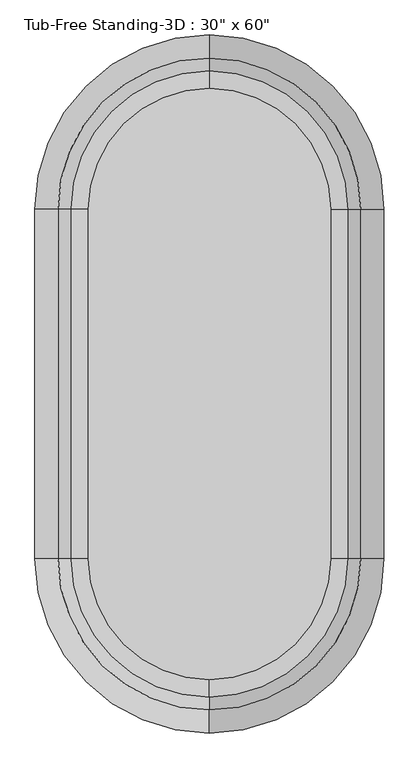
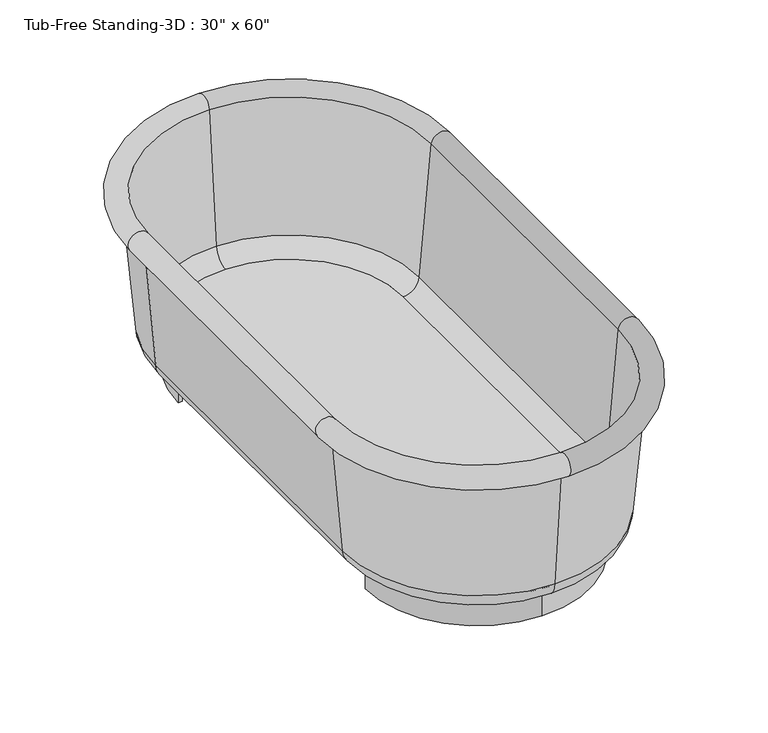
"""IFC4 building model written with IfcOpenShell, lengths in millimetres: flow terminal geometry."""

from ifc_helpers import new_model, si_unit, point, frame, frame_2d, origin, origin_with_axes, place, context, project, spatial, polyline, circle_curve, ellipse_curve, trimmed, segment, composite_curve, outline, extrude, source, transform, mapped, element, save
from ifc_brep_helpers import plane_surface, cylinder_surface, revolved_surface, advanced_brep


def flow_terminal_b374fae2(model_context):
    return source(origin(), model_context, "Body", "SolidModel", [
        extrude(outline(composite_curve([segment(trimmed(circle_curve(frame_2d((0.0, 381.0)), 254.0), [point((0.0, 635.0))], [point((-254.0, 381.0))], True, "CARTESIAN"), True, "CONTINUOUS"), segment(polyline([(-254.0, 381.0), (-264.2824236, 381.0)]), True, "CONTINUOUS"), segment(trimmed(circle_curve(frame_2d((0.0, 381.0)), 264.2824236), [point((-264.2824236, 381.0))], [point((0.0, 645.2824236))], False, "CARTESIAN"), True, "CONTINUOUS"), segment(trimmed(circle_curve(frame_2d((0.0, 381.0)), 264.2824236), [point((0.0, 645.2824236))], [point((264.2824236, 381.0))], False, "CARTESIAN"), True, "CONTINUOUS"), segment(polyline([(264.2824236, 381.0), (254.0, 381.0)]), True, "CONTINUOUS"), segment(trimmed(circle_curve(frame_2d((0.0, 381.0)), 254.0), [point((254.0, 381.0))], [point((0.0, 635.0))], True, "CARTESIAN"), True, "CONTINUOUS")], self_intersect=False)), origin_with_axes(), (0.0, 0.0, 1.0), 63.5),
        extrude(outline(composite_curve([segment(trimmed(circle_curve(frame_2d((0.0, -381.0)), 264.2824236), [point((0.0, -645.2824236))], [point((-264.2824236, -381.0))], False, "CARTESIAN"), True, "CONTINUOUS"), segment(polyline([(-264.2824236, -381.0), (-254.0, -381.0)]), True, "CONTINUOUS"), segment(trimmed(circle_curve(frame_2d((0.0, -381.0)), 254.0), [point((-254.0, -381.0))], [point((0.0, -635.0))], True, "CARTESIAN"), True, "CONTINUOUS"), segment(trimmed(circle_curve(frame_2d((0.0, -381.0)), 254.0), [point((0.0, -635.0))], [point((254.0, -381.0))], True, "CARTESIAN"), True, "CONTINUOUS"), segment(polyline([(254.0, -381.0), (264.2824236, -381.0)]), True, "CONTINUOUS"), segment(trimmed(circle_curve(frame_2d((0.0, -381.0)), 264.2824236), [point((264.2824236, -381.0))], [point((0.0, -645.2824236))], False, "CARTESIAN"), True, "CONTINUOUS")], self_intersect=False)), origin_with_axes(), (0.0, 0.0, 1.0), 63.5),
        extrude(outline(composite_curve([segment(polyline([(-264.2824236, -381.0), (-264.2824236, 381.0)]), True, "CONTINUOUS"), segment(trimmed(circle_curve(frame_2d((0.0, 381.0)), 264.2824236), [point((-264.2824236, 381.0))], [point((0.0, 645.2824236))], False, "CARTESIAN"), True, "CONTINUOUS"), segment(trimmed(circle_curve(frame_2d((0.0, 381.0)), 264.2824236), [point((0.0, 645.2824236))], [point((264.2824236, 381.0))], False, "CARTESIAN"), True, "CONTINUOUS"), segment(polyline([(264.2824236, 381.0), (264.2824236, -381.0)]), True, "CONTINUOUS"), segment(trimmed(circle_curve(frame_2d((0.0, -381.0)), 264.2824236), [point((264.2824236, -381.0))], [point((0.0, -645.2824236))], False, "CARTESIAN"), True, "CONTINUOUS"), segment(trimmed(circle_curve(frame_2d((0.0, -381.0)), 264.2824236), [point((0.0, -645.2824236))], [point((-264.2824236, -381.0))], False, "CARTESIAN"), True, "CONTINUOUS")], self_intersect=False)), frame((0.0, 0.0, 63.5), z_axis=(0.0, 0.0, 1.0), x_axis=(1.0, 0.0, 0.0)), (0.0, 0.0, 1.0), 15.08125),
        advanced_brep(
        [(0.0, -723.9, 406.4), (342.9, -381.0, 406.4), (355.6, -381.0, 406.4), (0.0, -736.6, 406.4), (0.0, -698.1045038, 111.5561295), (317.1045038, -381.0, 111.5561295), (0.0, -645.2824236, 63.1536107), (264.2824236, -381.0, 63.1536107), (0.0, -645.2824236, 78.0774627), (264.2824236, -381.0, 78.0774627), (0.0, -683.2374416, 112.8568289), (302.2374416, -381.0, 112.8568289), (0.0, -711.4561556, 435.3982063), (330.4561556, -381.0, 435.3982063), (-342.9, -381.0, 406.4), (-355.6, -381.0, 406.4), (-317.1045038, -381.0, 111.5561295), (-264.2824236, -381.0, 63.1536107), (-264.2824236, -381.0, 78.0774627), (-302.2374416, -381.0, 112.8568289), (-330.4561556, -381.0, 435.3982063), (-355.6, 381.0, 406.4), (-342.9, 381.0, 406.4), (-317.1045038, 381.0, 111.5561295), (-264.2824236, 381.0, 63.1536107), (-264.2824236, 381.0, 78.0774627), (-302.2374416, 381.0, 112.8568289), (-330.4561556, 381.0, 435.3982063), (0.0, 723.9, 406.4), (0.0, 736.6, 406.4), (0.0, 698.1045038, 111.5561295), (0.0, 645.2824236, 63.1536107), (0.0, 645.2824236, 78.0774627), (0.0, 683.2374416, 112.8568289), (0.0, 711.4561556, 435.3982063), (342.9, 381.0, 406.4), (355.6, 381.0, 406.4), (317.1045038, 381.0, 111.5561295), (264.2824236, 381.0, 63.1536107), (264.2824236, 381.0, 78.0774627), (302.2374416, 381.0, 112.8568289), (330.4561556, 381.0, 435.3982063)],
        [
            (0, 1, circle_curve(frame((0.0, -381.0, 406.4), z_axis=(0.0, 0.0, 1.0), x_axis=(1.0, 0.0, 0.0)), 342.9)),
            (1, 2),
            (2, 3, circle_curve(frame((0.0, -381.0, 406.4), z_axis=(0.0, 0.0, -1.0), x_axis=(1.0, 0.0, 0.0)), 355.6)),
            (3, 0),
            (4, 5, circle_curve(frame((0.0, -381.0, 111.5561295), z_axis=(0.0, 0.0, 1.0), x_axis=(1.0, 0.0, 0.0)), 317.1045038)),
            (5, 1),
            (0, 4),
            (6, 7, circle_curve(frame((0.0, -381.0, 63.1536107), z_axis=(0.0, 0.0, 1.0), x_axis=(1.0, 0.0, 0.0)), 264.2824236)),
            (7, 5, circle_curve(frame((264.2824236, -381.0, 116.1774627), z_axis=(0.0, -1.0, 0.0), x_axis=(1.0, 0.0, 0.0)), 53.023852)),
            (4, 6, circle_curve(frame((0.0, -645.2824236, 116.1774627), z_axis=(1.0, 0.0, 0.0), x_axis=(0.0, -1.0, 0.0)), 53.023852)),
            (8, 9, circle_curve(frame((0.0, -381.0, 78.0774627), z_axis=(0.0, 0.0, 1.0), x_axis=(1.0, 0.0, 0.0)), 264.2824236)),
            (9, 7),
            (6, 8),
            (10, 11, circle_curve(frame((0.0, -381.0, 112.8568289), z_axis=(0.0, 0.0, 1.0), x_axis=(1.0, 0.0, 0.0)), 302.2374416)),
            (11, 9, circle_curve(frame((264.2824236, -381.0, 116.1774627), z_axis=(0.0, 1.0, 0.0), x_axis=(1.0, 0.0, 0.0)), 38.1)),
            (8, 10, circle_curve(frame((0.0, -645.2824236, 116.1774627), z_axis=(-1.0, 0.0, 0.0), x_axis=(0.0, -1.0, 0.0)), 38.1)),
            (12, 13, circle_curve(frame((0.0, -381.0, 435.3982063), z_axis=(0.0, 0.0, 1.0), x_axis=(1.0, 0.0, 0.0)), 330.4561556)),
            (13, 11),
            (10, 12),
            (2, 13, circle_curve(frame((355.6, -381.0, 431.8), z_axis=(0.0, -1.0, 0.0), x_axis=(1.0, 0.0, 0.0)), 25.4)),
            (12, 3, circle_curve(frame((0.0, -736.6, 431.8), z_axis=(1.0, 0.0, 0.0), x_axis=(0.0, -1.0, 0.0)), 25.4)),
            (14, 0, circle_curve(frame((0.0, -381.0, 406.4), z_axis=(0.0, 0.0, 1.0), x_axis=(0.0, -1.0, 0.0)), 342.9)),
            (3, 15, circle_curve(frame((0.0, -381.0, 406.4), z_axis=(0.0, 0.0, -1.0), x_axis=(0.0, -1.0, 0.0)), 355.6)),
            (15, 14),
            (16, 4, circle_curve(frame((0.0, -381.0, 111.5561295), z_axis=(0.0, 0.0, 1.0), x_axis=(0.0, -1.0, 0.0)), 317.1045038)),
            (14, 16),
            (17, 6, circle_curve(frame((0.0, -381.0, 63.1536107), z_axis=(0.0, 0.0, 1.0), x_axis=(0.0, -1.0, 0.0)), 264.2824236)),
            (16, 17, circle_curve(frame((-264.2824236, -381.0, 116.1774627), z_axis=(0.0, -1.0, 0.0), x_axis=(-1.0, 0.0, 0.0)), 53.023852)),
            (18, 8, circle_curve(frame((0.0, -381.0, 78.0774627), z_axis=(0.0, 0.0, 1.0), x_axis=(0.0, -1.0, 0.0)), 264.2824236)),
            (17, 18),
            (19, 10, circle_curve(frame((0.0, -381.0, 112.8568289), z_axis=(0.0, 0.0, 1.0), x_axis=(0.0, -1.0, 0.0)), 302.2374416)),
            (18, 19, circle_curve(frame((-264.2824236, -381.0, 116.1774627), z_axis=(0.0, 1.0, 0.0), x_axis=(-1.0, 0.0, 0.0)), 38.1)),
            (20, 12, circle_curve(frame((0.0, -381.0, 435.3982063), z_axis=(0.0, 0.0, 1.0), x_axis=(0.0, -1.0, 0.0)), 330.4561556)),
            (19, 20),
            (20, 15, circle_curve(frame((-355.6, -381.0, 431.8), z_axis=(0.0, -1.0, 0.0), x_axis=(-1.0, 0.0, 0.0)), 25.4)),
            (15, 21),
            (21, 22),
            (22, 14),
            (22, 23),
            (23, 16),
            (23, 24, circle_curve(frame((-264.2824236, 381.0, 116.1774627), z_axis=(0.0, -1.0, 0.0), x_axis=(-1.0, 0.0, 0.0)), 53.023852)),
            (24, 17),
            (24, 25),
            (25, 18),
            (25, 26, circle_curve(frame((-264.2824236, 381.0, 116.1774627), z_axis=(0.0, 1.0, 0.0), x_axis=(-1.0, 0.0, 0.0)), 38.1)),
            (26, 19),
            (26, 27),
            (27, 20),
            (27, 21, circle_curve(frame((-355.6, 381.0, 431.8), z_axis=(0.0, -1.0, 0.0), x_axis=(-1.0, 0.0, 0.0)), 25.4)),
            (28, 22, circle_curve(frame((0.0, 381.0, 406.4), z_axis=(0.0, 0.0, 1.0), x_axis=(-1.0, 0.0, 0.0)), 342.9)),
            (21, 29, circle_curve(frame((0.0, 381.0, 406.4), z_axis=(0.0, 0.0, -1.0), x_axis=(-1.0, 0.0, 0.0)), 355.6)),
            (29, 28),
            (30, 23, circle_curve(frame((0.0, 381.0, 111.5561295), z_axis=(0.0, 0.0, 1.0), x_axis=(-1.0, 0.0, 0.0)), 317.1045038)),
            (28, 30),
            (31, 24, circle_curve(frame((0.0, 381.0, 63.1536107), z_axis=(0.0, 0.0, 1.0), x_axis=(-1.0, 0.0, 0.0)), 264.2824236)),
            (30, 31, circle_curve(frame((0.0, 645.2824236, 116.1774627), z_axis=(-1.0, 0.0, 0.0), x_axis=(0.0, 1.0, 0.0)), 53.023852)),
            (32, 25, circle_curve(frame((0.0, 381.0, 78.0774627), z_axis=(0.0, 0.0, 1.0), x_axis=(-1.0, 0.0, 0.0)), 264.2824236)),
            (31, 32),
            (33, 26, circle_curve(frame((0.0, 381.0, 112.8568289), z_axis=(0.0, 0.0, 1.0), x_axis=(-1.0, 0.0, 0.0)), 302.2374416)),
            (32, 33, circle_curve(frame((0.0, 645.2824236, 116.1774627), z_axis=(1.0, 0.0, 0.0), x_axis=(0.0, 1.0, 0.0)), 38.1)),
            (34, 27, circle_curve(frame((0.0, 381.0, 435.3982063), z_axis=(0.0, 0.0, 1.0), x_axis=(-1.0, 0.0, 0.0)), 330.4561556)),
            (33, 34),
            (34, 29, circle_curve(frame((0.0, 736.6, 431.8), z_axis=(-1.0, 0.0, 0.0), x_axis=(0.0, 1.0, 0.0)), 25.4)),
            (35, 28, circle_curve(frame((0.0, 381.0, 406.4), z_axis=(0.0, 0.0, 1.0), x_axis=(0.0, 1.0, 0.0)), 342.9)),
            (29, 36, circle_curve(frame((0.0, 381.0, 406.4), z_axis=(0.0, 0.0, -1.0), x_axis=(0.0, 1.0, 0.0)), 355.6)),
            (36, 35),
            (37, 30, circle_curve(frame((0.0, 381.0, 111.5561295), z_axis=(0.0, 0.0, 1.0), x_axis=(0.0, 1.0, 0.0)), 317.1045038)),
            (35, 37),
            (38, 31, circle_curve(frame((0.0, 381.0, 63.1536107), z_axis=(0.0, 0.0, 1.0), x_axis=(0.0, 1.0, 0.0)), 264.2824236)),
            (37, 38, circle_curve(frame((264.2824236, 381.0, 116.1774627), z_axis=(0.0, 1.0, 0.0), x_axis=(1.0, 0.0, 0.0)), 53.023852)),
            (39, 32, circle_curve(frame((0.0, 381.0, 78.0774627), z_axis=(0.0, 0.0, 1.0), x_axis=(0.0, 1.0, 0.0)), 264.2824236)),
            (38, 39),
            (40, 33, circle_curve(frame((0.0, 381.0, 112.8568289), z_axis=(0.0, 0.0, 1.0), x_axis=(0.0, 1.0, 0.0)), 302.2374416)),
            (39, 40, circle_curve(frame((264.2824236, 381.0, 116.1774627), z_axis=(0.0, -1.0, 0.0), x_axis=(1.0, 0.0, 0.0)), 38.1)),
            (41, 34, circle_curve(frame((0.0, 381.0, 435.3982063), z_axis=(0.0, 0.0, 1.0), x_axis=(0.0, 1.0, 0.0)), 330.4561556)),
            (40, 41),
            (41, 36, circle_curve(frame((355.6, 381.0, 431.8), z_axis=(0.0, 1.0, 0.0), x_axis=(1.0, 0.0, 0.0)), 25.4)),
            (36, 2),
            (1, 35),
            (5, 37),
            (7, 38),
            (9, 39),
            (11, 40),
            (13, 41),
        ],
        [
            plane_surface(frame((0.0, -381.0, 406.4), z_axis=(0.0, 0.0, -1.0), x_axis=(1.0, 0.0, 0.0))),
            revolved_surface(polyline([(342.9, -381.0, 406.4), (317.1045038, -381.0, 111.5561295)]), (0.0, -381.0, 431.8), (0.0, 0.0, -1.0)),
            revolved_surface(trimmed(ellipse_curve(frame((264.2824236, -381.0, 116.1774627), z_axis=(0.0, 1.0, 0.0), x_axis=(1.0, 0.0, 0.0)), 53.023852, 53.023852), [point((317.1045038, -381.0, 111.5561295))], [point((264.2824236, -381.0, 63.1536107))], True, "CARTESIAN"), (0.0, -381.0, 431.8), (0.0, 0.0, -1.0)),
            revolved_surface(polyline([(264.2824236, -381.0, 63.1536107), (264.2824236, -381.0, 78.07746270000001)]), (0.0, -381.0, 431.8), (0.0, 0.0, -1.0)),
            revolved_surface(trimmed(ellipse_curve(frame((264.2824236, -381.0, 116.1774627), z_axis=(0.0, -1.0, 0.0), x_axis=(1.0, 0.0, 0.0)), 38.1, 38.1), [point((264.2824236, -381.0, 78.0774627))], [point((302.2374416, -381.0, 112.8568289))], True, "CARTESIAN"), (0.0, -381.0, 431.8), (0.0, 0.0, -1.0)),
            revolved_surface(polyline([(302.2374416, -381.0, 112.8568289), (330.4561556, -381.0, 435.3982063)]), (0.0, -381.0, 431.8), (0.0, 0.0, -1.0)),
            revolved_surface(trimmed(ellipse_curve(frame((355.6, -381.0, 431.8), z_axis=(0.0, 1.0, 0.0), x_axis=(1.0, 0.0, 0.0)), 25.4, 25.4), [point((330.4561556, -381.0, 435.3982063))], [point((355.6, -381.0, 406.4))], True, "CARTESIAN"), (0.0, -381.0, 431.8), (0.0, 0.0, -1.0)),
            plane_surface(frame((0.0, -381.0, 406.4), z_axis=(0.0, 0.0, -1.0), x_axis=(0.0, -1.0, 0.0))),
            revolved_surface(polyline([(0.0, -723.9, 406.4), (0.0, -698.1045038, 111.5561295)]), (0.0, -381.0, 431.8), (0.0, 0.0, -1.0)),
            revolved_surface(trimmed(ellipse_curve(frame((0.0, -645.2824236, 116.1774627), z_axis=(1.0, 0.0, 0.0), x_axis=(0.0, -1.0, 0.0)), 53.023852, 53.023852), [point((0.0, -698.1045038, 111.5561295))], [point((0.0, -645.2824236, 63.1536107))], True, "CARTESIAN"), (0.0, -381.0, 431.8), (0.0, 0.0, -1.0)),
            revolved_surface(polyline([(0.0, -645.2824236, 63.1536107), (0.0, -645.2824236, 78.07746270000001)]), (0.0, -381.0, 431.8), (0.0, 0.0, -1.0)),
            revolved_surface(trimmed(ellipse_curve(frame((0.0, -645.2824236, 116.1774627), z_axis=(-1.0, 0.0, 0.0), x_axis=(0.0, -1.0, 0.0)), 38.1, 38.1), [point((0.0, -645.2824236, 78.0774627))], [point((0.0, -683.2374416, 112.8568289))], True, "CARTESIAN"), (0.0, -381.0, 431.8), (0.0, 0.0, -1.0)),
            revolved_surface(polyline([(0.0, -683.2374416, 112.8568289), (0.0, -711.4561556, 435.3982063)]), (0.0, -381.0, 431.8), (0.0, 0.0, -1.0)),
            revolved_surface(trimmed(ellipse_curve(frame((0.0, -736.6, 431.8), z_axis=(1.0, 0.0, 0.0), x_axis=(0.0, -1.0, 0.0)), 25.4, 25.4), [point((0.0, -711.4561556, 435.3982063))], [point((0.0, -736.6, 406.4))], True, "CARTESIAN"), (0.0, -381.0, 431.8), (0.0, 0.0, -1.0)),
            plane_surface(frame((-355.6, -381.0, 406.4), z_axis=(0.0, 0.0, -1.0), x_axis=(0.0, 1.0, 0.0))),
            plane_surface(frame((-342.9, -381.0, 406.4), z_axis=(-0.9961946980917455, 0.0, -0.08715574274765871), x_axis=(0.0, 1.0, 0.0))),
            cylinder_surface(frame((-264.2824236, -381.0, 116.1774627), z_axis=(0.0, -1.0, 0.0), x_axis=(-1.0, 0.0, 0.0)), 53.023852),
            plane_surface(frame((-264.2824236, -381.0, 63.1536107), z_axis=(1.0, 0.0, 0.0), x_axis=(0.0, 1.0, 0.0))),
            revolved_surface(polyline([(-302.38242360000004, 381.0, 116.1774627), (-302.38242360000004, -381.0, 116.1774627)]), (-264.2824236, -381.0, 116.1774627), (0.0, 1.0, 0.0)),
            plane_surface(frame((-302.2374416, -381.0, 112.8568289), z_axis=(0.9961946980917458, 0.0, 0.08715574274765651), x_axis=(0.0, 1.0, 0.0))),
            cylinder_surface(frame((-355.6, -381.0, 431.8), z_axis=(0.0, -1.0, 0.0), x_axis=(-1.0, 0.0, 0.0)), 25.4),
            plane_surface(frame((0.0, 381.0, 406.4), z_axis=(0.0, 0.0, -1.0), x_axis=(-1.0, 0.0, 0.0))),
            revolved_surface(polyline([(-342.9, 381.0, 406.4), (-317.1045038, 381.0, 111.5561295)]), (0.0, 381.0, 431.8), (0.0, 0.0, -1.0)),
            revolved_surface(trimmed(ellipse_curve(frame((-264.2824236, 381.0, 116.1774627), z_axis=(0.0, -1.0, 0.0), x_axis=(-1.0, 0.0, 0.0)), 53.023852, 53.023852), [point((-317.1045038, 381.0, 111.5561295))], [point((-264.2824236, 381.0, 63.1536107))], True, "CARTESIAN"), (0.0, 381.0, 431.8), (0.0, 0.0, -1.0)),
            revolved_surface(polyline([(-264.2824236, 381.0, 63.1536107), (-264.2824236, 381.0, 78.07746270000001)]), (0.0, 381.0, 431.8), (0.0, 0.0, -1.0)),
            revolved_surface(trimmed(ellipse_curve(frame((-264.2824236, 381.0, 116.1774627), z_axis=(0.0, 1.0, 0.0), x_axis=(-1.0, 0.0, 0.0)), 38.1, 38.1), [point((-264.2824236, 381.0, 78.0774627))], [point((-302.2374416, 381.0, 112.8568289))], True, "CARTESIAN"), (0.0, 381.0, 431.8), (0.0, 0.0, -1.0)),
            revolved_surface(polyline([(-302.2374416, 381.0, 112.8568289), (-330.4561556, 381.0, 435.3982063)]), (0.0, 381.0, 431.8), (0.0, 0.0, -1.0)),
            revolved_surface(trimmed(ellipse_curve(frame((-355.6, 381.0, 431.8), z_axis=(0.0, -1.0, 0.0), x_axis=(-1.0, 0.0, 0.0)), 25.4, 25.4), [point((-330.4561556, 381.0, 435.3982063))], [point((-355.6, 381.0, 406.4))], True, "CARTESIAN"), (0.0, 381.0, 431.8), (0.0, 0.0, -1.0)),
            plane_surface(frame((0.0, 381.0, 406.4), z_axis=(0.0, 0.0, -1.0), x_axis=(0.0, 1.0, 0.0))),
            revolved_surface(polyline([(0.0, 723.9, 406.4), (0.0, 698.1045038, 111.5561295)]), (0.0, 381.0, 431.8), (0.0, 0.0, -1.0)),
            revolved_surface(trimmed(ellipse_curve(frame((0.0, 645.2824236, 116.1774627), z_axis=(-1.0, 0.0, 0.0), x_axis=(0.0, 1.0, 0.0)), 53.023852, 53.023852), [point((0.0, 698.1045038, 111.5561295))], [point((0.0, 645.2824236, 63.1536107))], True, "CARTESIAN"), (0.0, 381.0, 431.8), (0.0, 0.0, -1.0)),
            revolved_surface(polyline([(0.0, 645.2824236, 63.1536107), (0.0, 645.2824236, 78.07746270000001)]), (0.0, 381.0, 431.8), (0.0, 0.0, -1.0)),
            revolved_surface(trimmed(ellipse_curve(frame((0.0, 645.2824236, 116.1774627), z_axis=(1.0, 0.0, 0.0), x_axis=(0.0, 1.0, 0.0)), 38.1, 38.1), [point((0.0, 645.2824236, 78.0774627))], [point((0.0, 683.2374416, 112.8568289))], True, "CARTESIAN"), (0.0, 381.0, 431.8), (0.0, 0.0, -1.0)),
            revolved_surface(polyline([(0.0, 683.2374416, 112.8568289), (0.0, 711.4561556, 435.3982063)]), (0.0, 381.0, 431.8), (0.0, 0.0, -1.0)),
            revolved_surface(trimmed(ellipse_curve(frame((0.0, 736.6, 431.8), z_axis=(-1.0, 0.0, 0.0), x_axis=(0.0, 1.0, 0.0)), 25.4, 25.4), [point((0.0, 711.4561556, 435.3982063))], [point((0.0, 736.6, 406.4))], True, "CARTESIAN"), (0.0, 381.0, 431.8), (0.0, 0.0, -1.0)),
            plane_surface(frame((355.6, 381.0, 406.4), z_axis=(0.0, 0.0, -1.0), x_axis=(0.0, -1.0, 0.0))),
            plane_surface(frame((342.9, 381.0, 406.4), z_axis=(0.9961946980917455, 0.0, -0.08715574274765871), x_axis=(0.0, -1.0, 0.0))),
            cylinder_surface(frame((264.2824236, 381.0, 116.1774627), z_axis=(0.0, 1.0, 0.0), x_axis=(1.0, 0.0, 0.0)), 53.023852),
            plane_surface(frame((264.2824236, 381.0, 63.1536107), z_axis=(-1.0, 0.0, 0.0), x_axis=(0.0, -1.0, 0.0))),
            revolved_surface(polyline([(302.38242360000004, -381.0, 116.1774627), (302.38242360000004, 381.0, 116.1774627)]), (264.2824236, 381.0, 116.1774627), (0.0, -1.0, 0.0)),
            plane_surface(frame((302.2374416, 381.0, 112.8568289), z_axis=(-0.9961946980917458, 0.0, 0.08715574274765651), x_axis=(0.0, -1.0, 0.0))),
            cylinder_surface(frame((355.6, 381.0, 431.8), z_axis=(0.0, 1.0, 0.0), x_axis=(1.0, 0.0, 0.0)), 25.4),
        ],
        [
            (0, [[1, 2, 3, 4]]),
            (1, [[5, 6, -1, 7]]),
            (2, [[8, 9, -5, 10]]),
            (3, [[11, 12, -8, 13]]),
            (4, [[14, 15, -11, 16]]),
            (5, [[17, 18, -14, 19]]),
            (6, [[-3, 20, -17, 21]]),
            (7, [[22, -4, 23, 24]]),
            (8, [[25, -7, -22, 26]]),
            (9, [[27, -10, -25, 28]]),
            (10, [[29, -13, -27, 30]]),
            (11, [[31, -16, -29, 32]]),
            (12, [[33, -19, -31, 34]]),
            (13, [[-23, -21, -33, 35]]),
            (14, [[-24, 36, 37, 38]]),
            (15, [[-26, -38, 39, 40]]),
            (16, [[-28, -40, 41, 42]]),
            (17, [[-30, -42, 43, 44]]),
            (18, [[-32, -44, 45, 46]]),
            (19, [[-34, -46, 47, 48]]),
            (20, [[-35, -48, 49, -36]]),
            (21, [[50, -37, 51, 52]]),
            (22, [[53, -39, -50, 54]]),
            (23, [[55, -41, -53, 56]]),
            (24, [[57, -43, -55, 58]]),
            (25, [[59, -45, -57, 60]]),
            (26, [[61, -47, -59, 62]]),
            (27, [[-51, -49, -61, 63]]),
            (28, [[64, -52, 65, 66]]),
            (29, [[67, -54, -64, 68]]),
            (30, [[69, -56, -67, 70]]),
            (31, [[71, -58, -69, 72]]),
            (32, [[73, -60, -71, 74]]),
            (33, [[75, -62, -73, 76]]),
            (34, [[-65, -63, -75, 77]]),
            (35, [[-66, 78, -2, 79]]),
            (36, [[-68, -79, -6, 80]]),
            (37, [[-70, -80, -9, 81]]),
            (38, [[-72, -81, -12, 82]]),
            (39, [[-74, -82, -15, 83]]),
            (40, [[-76, -83, -18, 84]]),
            (41, [[-77, -84, -20, -78]]),
        ],
    ),
    ])


if __name__ == "__main__":
    model = new_model("IFC4")
    model_context = context("Model", 3, world=origin())
    ifc_project = project(units=[si_unit("LENGTHUNIT", "METRE", prefix="MILLI")], contexts=[model_context])
    site = spatial("IfcSite", under=ifc_project)
    building = spatial("IfcBuilding", under=site)
    placement = place(None, origin())
    flow_terminal_shape = flow_terminal_b374fae2(model_context)
    element("IfcFlowTerminal", 1, ObjectType="Tub-Free Standing-3D : 30\" x 60\"", at=placement, inside=building, context=model_context, shape_type="MappedRepresentation", body=[
        mapped(flow_terminal_shape, transform((0.0, 0.0, 0.0), x_axis=(1.0, 0.0, 0.0), y_axis=(0.0, 1.0, 0.0), z_axis=(0.0, 0.0, 1.0))),
    ])
    save(model, "model.ifc")

# Revit data of these elements
# Type "Tub-Free Standing-3D : 30\" x 60\""
#   Assembly Code = "D2010110"
#   Height = 1' - 6"
#   Length = 5' - 0"
#   Width = 2' - 6"
#   Tub Material = Porcelain, Ivory
#   Default Elevation = 0
# Element 1 (IfcFlowTerminal, "Tub-Free Standing-3D : 30\" x 60\"")
#   Materials on its faces: "Porcelain, Ivory"
# Materials
#   "Porcelain, Ivory": class "Ceramic", colour RGB 247 247 239, transparency 0, Description = "Porcelain, ivory", Cost = 0
